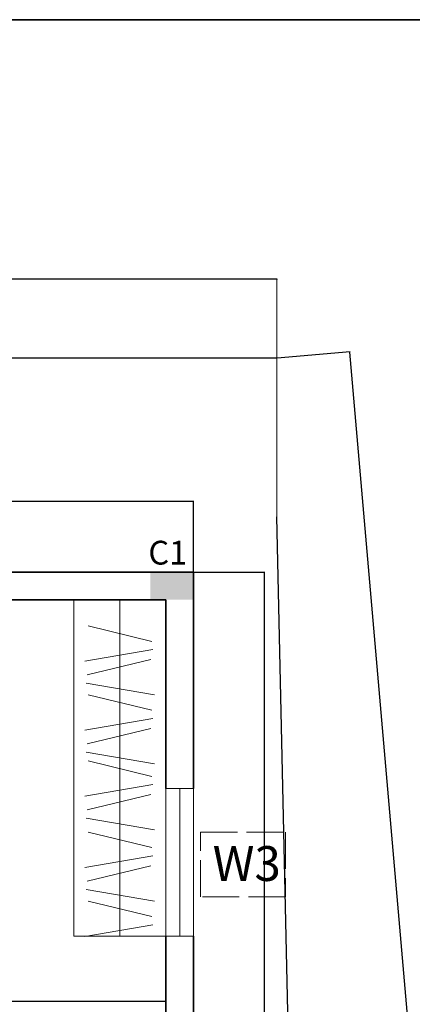
# Model space of a CAD drawing. Units: inches. Extents: x -269 to 4574, y -694 to 313.
# Tile 16 of 19: x 395 to 522, y -122 to 198. Entities that reach past the tile are written whole.
import ezdxf

# ---------------------------------------------------------------- set-up
doc = ezdxf.new("R2010")
doc.units = ezdxf.units.IN
doc.header["$MEASUREMENT"] = 0
doc.linetypes.add('ACAD_ISO02W100', pattern=[15, 12, -3])
for name, color, linetype, lineweight in [('A-ANNO-FRAM', 7, 'ACAD_ISO02W100', 13), ('A-ANNO-IDEN', 6, 'Continuous', 18), ('A-COLS', 5, 'Continuous', 35), ('A-COLS-IDEN', 6, 'Continuous', 18), ('A-FLOR-CASE', 2, 'Continuous', 18), ('BORDER', 7, 'Continuous', 35), ('C-PROP', 7, 'Continuous', 25), ('DIMENSION', 5, 'Continuous', 18), ('WALL', 1, 'Continuous', 35), ('WINDOWS', 2, 'Continuous', 18)]:
    doc.layers.add(name, color=color, linetype=linetype, lineweight=lineweight)
doc.dimstyles.get("Standard").update_dxf_attribs({"dimtxt": 10, "dimasz": 0.18, "dimexe": 0.18, "dimexo": 0.0625, "dimgap": 0.09, "dimtad": 0, "dimdec": 1, "dimzin": 0, "dimdsep": 46, "dimlunit": 3, "dimtxsty": 'Standard', "dimcen": 0.09, "dimclrt": 7, "dimadec": 0, "dimazin": 0, "dimtfac": 1, "dimtdec": 1, "dimtofl": 0, "dimtmove": 0, "dimatfit": 3, "dimfxl": 1, "dimtolj": 1, "dimtzin": 0, "dimarcsym": 0})

# ---------------------------------------------------------------- blocks, each defined once
blk = doc.blocks.new('*D1')
at = {"layer": 'Defpoints', "color": 0, "lineweight": 0, "transparency": 16777216}
for p in [(451.14, 41.26), (7.14, 18.27), (451.14, 18.27)]:
    blk.add_point(p, dxfattribs=at)
at = {"layer": 'DIMENSION', "color": 0, "lineweight": -2, "transparency": 16777216}
for p, q in [((7.14, 18.33), (7.14, 41.44)), ((7.32, 41.26), (219.05, 41.26)), ((450.96, 41.26), (239.23, 41.26)), ((451.14, 18.33), (451.14, 41.44))]:
    blk.add_line(p, q, dxfattribs=at)
at = {"layer": 'DIMENSION', "color": 0, "lineweight": 0, "transparency": 16777216}
for points in [[(7.32, 41.29), (7.32, 41.23), (7.14, 41.26)], [(450.96, 41.29), (450.96, 41.23), (451.14, 41.26)]]:
    blk.add_solid(points, dxfattribs=at)
at = {"layer": 'DIMENSION', "color": 0, "transparency": 16777216, "insert": (229.14, 41.26), "char_height": 10, "attachment_point": 5}
blk.add_mtext("\\A1;37'", dxfattribs=at)
blk = doc.blocks.new('*D20')
at = {"layer": 'Defpoints', "color": 0, "lineweight": 0, "transparency": 16777216}
for p in [(442.14, -121.56), (262.14, -122.44), (442.14, -122.44)]:
    blk.add_point(p, dxfattribs=at)
at = {"layer": 'DIMENSION', "color": 0, "lineweight": -2, "transparency": 16777216}
for p, q in [((262.14, -122.38), (262.14, -121.38)), ((262.32, -121.56), (343, -121.56)), ((441.96, -121.56), (361.27, -121.56)), ((442.14, -122.38), (442.14, -121.38))]:
    blk.add_line(p, q, dxfattribs=at)
at = {"layer": 'DIMENSION', "color": 0, "lineweight": 0, "transparency": 16777216}
for points in [[(262.32, -121.53), (262.32, -121.59), (262.14, -121.56)], [(441.96, -121.53), (441.96, -121.59), (442.14, -121.56)]]:
    blk.add_solid(points, dxfattribs=at)
at = {"layer": 'DIMENSION', "color": 0, "transparency": 16777216, "insert": (352.14, -121.56), "char_height": 10, "attachment_point": 5}
blk.add_mtext("\\A1;15'", dxfattribs=at)
blk = doc.blocks.new('*D27')
at = {"layer": 'Defpoints', "color": 0, "lineweight": 0, "transparency": 16777216}
for p in [(451.14, 18.27), (451.14, -365.73), (474.13, -365.73)]:
    blk.add_point(p, dxfattribs=at)
at = {"layer": 'DIMENSION', "color": 0, "lineweight": -2, "transparency": 16777216}
for p, q in [((451.2, 18.27), (474.31, 18.27)), ((474.13, 18.09), (474.13, -163.64)), ((474.13, -365.55), (474.13, -183.82)), ((451.2, -365.73), (474.31, -365.73))]:
    blk.add_line(p, q, dxfattribs=at)
at = {"layer": 'DIMENSION', "color": 0, "lineweight": 0, "transparency": 16777216}
for points in [[(474.1, 18.09), (474.16, 18.09), (474.13, 18.27)], [(474.1, -365.55), (474.16, -365.55), (474.13, -365.73)]]:
    blk.add_solid(points, dxfattribs=at)
at = {"layer": 'DIMENSION', "color": 0, "transparency": 16777216, "insert": (474.13, -173.73), "char_height": 10, "attachment_point": 5, "rotation": 90}
blk.add_mtext("\\A1;32'", dxfattribs=at)
blk = doc.blocks.new('*D32')
at = {"layer": 'Defpoints', "color": 0, "lineweight": 0, "transparency": 16777216}
for p in [(-37.71, 113.85), (478.29, 113.67), (478.29, 113.64)]:
    blk.add_point(p, dxfattribs=at)
at = {"layer": 'DIMENSION', "color": 0, "lineweight": -2, "transparency": 16777216}
for p, q in [((-37.71, 113.79), (-37.71, 113.46)), ((-37.53, 113.64), (210.2, 113.64)), ((478.11, 113.64), (230.38, 113.64)), ((478.29, 113.61), (478.29, 113.46))]:
    blk.add_line(p, q, dxfattribs=at)
at = {"layer": 'DIMENSION', "color": 0, "lineweight": 0, "transparency": 16777216}
for points in [[(-37.53, 113.67), (-37.53, 113.61), (-37.71, 113.64)], [(478.11, 113.67), (478.11, 113.61), (478.29, 113.64)]]:
    blk.add_solid(points, dxfattribs=at)
at = {"layer": 'DIMENSION', "color": 0, "transparency": 16777216, "insert": (220.29, 113.64), "char_height": 10, "attachment_point": 5}
blk.add_mtext("\\A1;43'", dxfattribs=at)
blk = doc.blocks.new('*D35')
at = {"layer": 'Defpoints', "color": 0, "lineweight": 0, "transparency": 16777216}
for p in [(478.29, 88), (551.23, -476.8), (527.63, -478.86)]:
    blk.add_point(p, dxfattribs=at)
at = {"layer": 'DIMENSION', "color": 0, "lineweight": -2, "transparency": 16777216}
for p, q in [((478.36, 88.01), (502.07, 90.07)), ((501.91, 89.87), (523.81, -161.74)), ((551.21, -476.62), (529.31, -225.01)), ((527.69, -478.85), (551.41, -476.79))]:
    blk.add_line(p, q, dxfattribs=at)
at = {"layer": 'DIMENSION', "color": 0, "lineweight": 0, "transparency": 16777216}
for points in [[(501.94, 89.88), (501.88, 89.87), (501.89, 90.05)], [(551.24, -476.62), (551.18, -476.63), (551.23, -476.8)]]:
    blk.add_solid(points, dxfattribs=at)
at = {"layer": 'DIMENSION', "color": 0, "transparency": 16777216, "insert": (526.56, -193.38), "char_height": 10, "attachment_point": 5, "rotation": 274.9738}
blk.add_mtext('\\A1;47\'-5.0"', dxfattribs=at)
blk = doc.blocks.new('GLAZ-48IN')
blk.add_line((4.5, 0), (4.5, 48))
blk.add_lwpolyline([(0, 48), (9, 48), (9, 0), (0, 0)], close=True)
blk = doc.blocks.new('COLUMN-9x14-PLAN')
h = blk.add_hatch(color=256)
h.dxf.hatch_style = 1
h.paths.add_polyline_path([(9, 14), (0, 14), (0, 0), (9, 0), (9, 5)])

msp = doc.modelspace()

# ---------------------------------------------------------------- linework, layer by layer
at = {"layer": 'A-ANNO-FRAM'}
msp.add_lwpolyline([(453.42, -66.41), (481.03, -66.41), (481.03, -87.52), (453.42, -87.52)], close=True, dxfattribs=at)
at = {"layer": 'A-FLOR-CASE'}
for p, q in [((412.14, 9.27), (412.14, -100.23)), ((427.14, -100.23), (427.14, 9.27)), ((416.81, 0.74), (437.59, -4.3)), ((415.72, -10.78), (437.95, -6.99)), ((437.3, -10.19), (416.52, -15.24)), ((438.39, -21.71), (416.16, -17.92)), ((416.81, -21.71), (437.59, -26.75)), ((415.72, -33.22), (437.95, -29.43)), ((437.3, -32.64), (416.52, -37.68)), ((438.39, -44.15), (416.16, -40.36)), ((416.81, -43.21), (437.59, -48.25)), ((415.72, -54.72), (437.95, -50.93)), ((437.3, -54.14), (416.52, -59.18)), ((438.39, -65.65), (416.16, -61.87)), ((416.81, -66.42), (437.59, -71.46)), ((415.72, -77.94), (437.95, -74.15)), ((437.3, -77.35), (416.52, -82.4)), ((438.39, -88.87), (416.16, -85.08)), ((416.81, -88.83), (437.59, -93.87)), ((415.72, -100.35), (437.95, -96.56)), ((442.14, -100.23), (412.14, -100.23))]:
    msp.add_line(p, q, dxfattribs=at)
at = {"layer": 'BORDER'}
msp.add_lwpolyline([(-268.51, 198.09), (666.62, 198.09), (666.62, -693.82), (-268.51, -693.82)], close=True, dxfattribs=at)
at = {"layer": 'C-PROP'}
for p, q in [((-37.71, 88), (478.29, 88)), ((490.29, -506.83), (478.29, 36.26))]:
    msp.add_line(p, q, dxfattribs=at)
at = {"layer": 'DIMENSION'}
msp.add_line((478.29, 36.32), (478.29, 113.85), dxfattribs=at)
msp.add_solid([(478.11, 113.7), (478.11, 113.64), (478.29, 113.67)], dxfattribs=at)
at = {"layer": 'WALL'}
for p, q in [((380.64, 18.27), (451.14, 18.27)), ((451.14, 18.27), (451.14, -52.23)), ((380.64, 9.27), (442.14, 9.27)), ((442.14, 9.27), (442.14, -52.23)), ((442.14, -100.23), (442.14, -170.73)), ((451.14, -100.23), (451.14, -208.23))]:
    msp.add_line(p, q, dxfattribs=at)

# ---------------------------------------------------------------- block references
at = {"layer": 'A-COLS', "rotation": 90.00000000000006}
msp.add_blockref('COLUMN-9x14-PLAN', (451.14, 9.27), dxfattribs=at)
at = {"layer": 'WINDOWS'}
msp.add_blockref('GLAZ-48IN', (442.14, -100.23), dxfattribs=at)

# ---------------------------------------------------------------- texts
at = {"layer": 'A-ANNO-IDEN'}
msp.add_text('W3', height=11.343, dxfattribs=at).set_placement((457.38, -82.3))
at = {"layer": 'A-COLS-IDEN'}
msp.add_text('C1', height=7.741, dxfattribs=at).set_placement((436.45, 20.7))

# ---------------------------------------------------------------- dimensions: what is measured, and where the dimension line sits
at = {"layer": 'DIMENSION'}
for base, p1, p2, picture, middle in [((478.29, 113.64), (-37.71, 113.85), (478.29, 113.67), '*D32', (220.29, 113.64)), ((451.14, 41.26), (7.14, 18.27), (451.14, 18.27), '*D1', (229.14, 41.26)), ((442.14, -121.56), (262.14, -122.44), (442.14, -122.44), '*D20', (352.14, -121.56))]:
    dim = msp.add_linear_dim(base=base, p1=p1, p2=p2, dimstyle='Standard', override={"dimclrd": 0, "dimclre": 0, "dimclrt": 0}, dxfattribs=at)
    dim.commit()
    dim.dimension.update_dxf_attribs({"geometry": picture, "text_midpoint": middle})
dim = msp.add_aligned_dim(p1=(478.29, 88), p2=(527.63, -478.86), distance=23.69, dimstyle='Standard', override={"dimclrd": 0, "dimclre": 0, "dimclrt": 0}, dxfattribs=at)
dim.commit()
dim.dimension.update_dxf_attribs({"geometry": '*D35', "text_midpoint": (526.56, -193.38)})
dim = msp.add_linear_dim(base=(474.13, -365.73), p1=(451.14, 18.27), p2=(451.14, -365.73), angle=90, dimstyle='Standard', override={"dimclrd": 0, "dimclre": 0, "dimclrt": 0}, dxfattribs=at)
dim.commit()
dim.dimension.update_dxf_attribs({"geometry": '*D27', "text_midpoint": (474.13, -173.73)})

doc.saveas('drawing.dxf')
